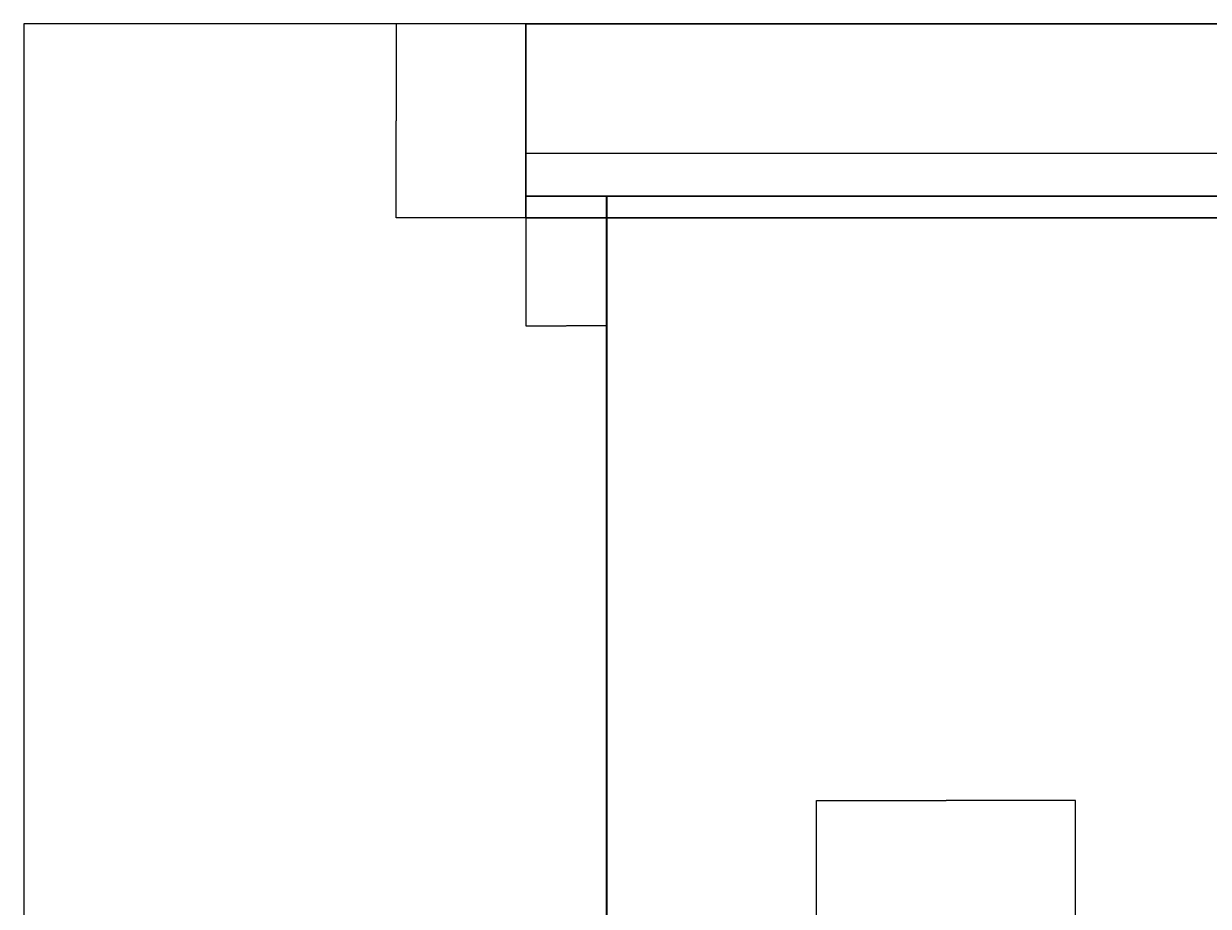
# Model space of a CAD drawing. Units: millimetres. Extents: x 54 to 12356, y 76 to 11627.
# Tile 1 of 2: x 54 to 5541, y 6935 to 11026. Entities that reach past the tile are written whole.
import ezdxf

# ---------------------------------------------------------------- set-up
doc = ezdxf.new("R2010")
doc.units = ezdxf.units.MM
for name, color, linetype, lineweight in [('A-ANNO-DIMS', 2, 'Continuous', 18), ('A-ROOF', 7, 'Continuous', 30), ('A-WALL', 7, 'Continuous', 35)]:
    doc.layers.add(name, color=color, linetype=linetype, lineweight=lineweight)
doc.styles.get("Standard").update_dxf_attribs({"font": 'arial.ttf'})
doc.dimstyles.get("Standard").update_dxf_attribs({"dimtxt": 0.18, "dimasz": 0.18, "dimexe": 0.18, "dimexo": 0.0625, "dimgap": 0.09, "dimtad": 0, "dimtih": 1, "dimtoh": 1, "dimdec": 4, "dimzin": 0, "dimdsep": 46, "dimtxsty": 'Standard', "dimcen": 0.09, "dimadec": 0, "dimazin": 0, "dimtfac": 1, "dimtdec": 4, "dimtofl": 0, "dimtmove": 0, "dimatfit": 3, "dimfxl": 1, "dimtolj": 1, "dimtzin": 0, "dimarcsym": 0})

# ---------------------------------------------------------------- blocks, each defined once
blk = doc.blocks.new('*D20')
at = {"layer": 'A-ANNO-DIMS', "color": 0, "lineweight": -2, "transparency": 16777216}
for p, q in [((2379.868777000001, 11026.423357), (54.25127699999922, 11026.423357)), ((54.43127699999891, 11026.243357), (54.43127700000006, 5851.605321529333)), ((54.43127700000121, 676.6033570000001), (54.43127700000006, 5851.24139247067)), ((654.8687770000003, 676.4233570000002), (54.2512770000013, 676.4233570000001))]:
    blk.add_line(p, q, dxfattribs=at)
at = {"layer": 'A-ANNO-DIMS', "color": 0, "transparency": 16777216}
for points in [[(54.40127699999891, 11026.243357), (54.46127699999891, 11026.243357), (54.43127699999891, 11026.423357)], [(54.40127700000121, 676.6033570000001), (54.46127700000121, 676.6033570000001), (54.43127700000121, 676.4233570000001)]]:
    blk.add_solid(points, dxfattribs=at)
at = {"layer": 'Defpoints', "color": 0, "transparency": 16777216}
for p in [(54.43127699999891, 11026.423357), (2379.931277000001, 11026.423357), (654.9312770000003, 676.4233570000002)]:
    blk.add_point(p, dxfattribs=at)
at = {"layer": 'A-ANNO-DIMS', "color": 0, "transparency": 16777216, "insert": (54.4312770000017, 5851.423357000001), "char_height": 0.18, "attachment_point": 5}
blk.add_mtext('\\A1;10350', dxfattribs=at)
blk = doc.blocks.new('*D21')
at = {"layer": 'A-ANNO-DIMS', "color": 0, "lineweight": -2, "transparency": 16777216}
for p, q in [((2379.931277, 11026.360857), (2379.931277, 10425.743357)), ((11379.931277, 11026.360857), (11379.931277, 10425.743357)), ((2380.111277, 10425.923357), (6879.57281178854, 10425.923357)), ((11379.751277, 10425.923357), (6880.289742211459, 10425.923357))]:
    blk.add_line(p, q, dxfattribs=at)
at = {"layer": 'A-ANNO-DIMS', "color": 0, "transparency": 16777216}
for points in [[(2380.111277, 10425.953357), (2380.111277, 10425.893357), (2379.931277, 10425.923357)], [(11379.751277, 10425.953357), (11379.751277, 10425.893357), (11379.931277, 10425.923357)]]:
    blk.add_solid(points, dxfattribs=at)
at = {"layer": 'Defpoints', "color": 0, "transparency": 16777216}
for p in [(2379.931277, 11026.423357), (11379.931277, 11026.423357), (2379.931277, 10425.923357)]:
    blk.add_point(p, dxfattribs=at)
at = {"layer": 'A-ANNO-DIMS', "color": 0, "transparency": 16777216, "insert": (6879.931277, 10425.923357), "char_height": 0.18, "attachment_point": 5}
blk.add_mtext('\\A1;9000', dxfattribs=at)
blk = doc.blocks.new('*D22')
at = {"layer": 'A-ANNO-DIMS', "color": 0, "lineweight": -2, "transparency": 16777216}
for p, q in [((2379.868777000001, 11026.423357), (1779.251277000001, 11026.423357)), ((1779.431277000001, 11026.243357), (1779.431277000002, 10576.60526013779)), ((1779.431277000002, 10126.603357), (1779.431277000002, 10576.24145386221)), ((2379.868777000001, 10126.423357), (1779.251277000001, 10126.423357))]:
    blk.add_line(p, q, dxfattribs=at)
at = {"layer": 'A-ANNO-DIMS', "color": 0, "transparency": 16777216}
for points in [[(1779.401277000001, 11026.243357), (1779.461277000001, 11026.243357), (1779.431277000001, 11026.423357)], [(1779.401277000002, 10126.603357), (1779.461277000002, 10126.603357), (1779.431277000002, 10126.423357)]]:
    blk.add_solid(points, dxfattribs=at)
at = {"layer": 'Defpoints', "color": 0, "transparency": 16777216}
for p in [(1779.431277000001, 11026.423357), (2379.931277000001, 11026.423357), (2379.931277000001, 10126.423357)]:
    blk.add_point(p, dxfattribs=at)
at = {"layer": 'A-ANNO-DIMS', "color": 0, "transparency": 16777216, "insert": (1779.431277000004, 10576.423357), "char_height": 0.18, "attachment_point": 5}
blk.add_mtext('\\A1;900', dxfattribs=at)
blk = doc.blocks.new('*D23')
at = {"layer": 'A-ANNO-DIMS', "color": 0, "lineweight": -2, "transparency": 16777216}
for p, q in [((2379.931277, 10226.360857), (2379.931277, 9625.743357)), ((2754.931277, 10226.360857), (2754.931277, 9625.743357)), ((2380.111277, 9625.923357), (2567.14181588131, 9625.923357)), ((2754.751277, 9625.923357), (2567.720738118691, 9625.923357))]:
    blk.add_line(p, q, dxfattribs=at)
at = {"layer": 'A-ANNO-DIMS', "color": 0, "transparency": 16777216}
for points in [[(2380.111277, 9625.953357), (2380.111277, 9625.893357), (2379.931277, 9625.923357)], [(2754.751277, 9625.953357), (2754.751277, 9625.893357), (2754.931277, 9625.923357)]]:
    blk.add_solid(points, dxfattribs=at)
at = {"layer": 'Defpoints', "color": 0, "transparency": 16777216}
for p in [(2379.931277, 10226.423357), (2754.931277, 10226.423357), (2379.931277, 9625.923357)]:
    blk.add_point(p, dxfattribs=at)
at = {"layer": 'A-ANNO-DIMS', "color": 0, "transparency": 16777216, "insert": (2567.431277, 9625.923357), "char_height": 0.18, "attachment_point": 5}
blk.add_mtext('\\A1;375', dxfattribs=at)
blk = doc.blocks.new('*D35')
at = {"layer": 'A-ANNO-DIMS', "color": 0, "lineweight": -2, "transparency": 16777216}
for p, q in [((3726.740342, 6825.348683), (3726.740342, 7425.966183000001)), ((3726.920342, 7425.786183000001), (4326.390348821282, 7425.786183000001)), ((4926.560342, 7425.786183000001), (4327.090335178717, 7425.786183000001)), ((4926.740342, 6825.348683), (4926.740342, 7425.966183000001))]:
    blk.add_line(p, q, dxfattribs=at)
at = {"layer": 'A-ANNO-DIMS', "color": 0, "transparency": 16777216}
for points in [[(3726.920342, 7425.816183000001), (3726.920342, 7425.756183), (3726.740342, 7425.786183000001)], [(4926.560342, 7425.816183000001), (4926.560342, 7425.756183), (4926.740342, 7425.786183000001)]]:
    blk.add_solid(points, dxfattribs=at)
at = {"layer": 'Defpoints', "color": 0, "transparency": 16777216}
for p in [(4926.740342, 7425.786183000001), (3726.740342, 6825.286183), (4926.740342, 6825.286183)]:
    blk.add_point(p, dxfattribs=at)
at = {"layer": 'A-ANNO-DIMS', "color": 0, "transparency": 16777216, "insert": (4326.740341999999, 7425.786183000001), "char_height": 0.18, "attachment_point": 5}
blk.add_mtext('\\A1;1200', dxfattribs=at)

msp = doc.modelspace()

# ---------------------------------------------------------------- linework, layer by layer
at = {"layer": 'A-ROOF'}
for p, q in [((2379.931277323882, 10126.42335733614), (2379.931277323882, 11026.42335733614)), ((2379.931277323882, 11026.42335733614), (11379.93127732388, 11026.42335733614)), ((2379.931277323883, 10826.42335733614), (2379.931277323883, 10726.42335733614)), ((11379.93127732388, 10226.42335733614), (2379.931277323882, 10226.42335733614)), ((2379.931277323882, 10126.42335733614), (11004.93127732388, 10126.42335733614))]:
    msp.add_line(p, q, dxfattribs=at)
at = {"layer": 'A-WALL'}
msp.add_line((2754.931277323886, 1276.42335733614), (2754.931277323885, 10226.42335733614), dxfattribs=at)

# ---------------------------------------------------------------- dimensions: what is measured, and where the dimension line sits
at = {"layer": 'A-ANNO-DIMS'}
for base, p1, p2, angle, picture, middle in [((54.43127699999891, 11026.423357), (654.931277, 676.423357), (2379.931277, 11026.423357), 90, '*D20', (54.4312770000017, 5851.423357000001)), ((1779.431277000001, 11026.423357), (2379.931277, 10126.423357), (2379.931277, 11026.423357), 90, '*D22', (1779.431277000004, 10576.423357)), ((2379.931277, 10425.923357), (11379.931277, 11026.423357), (2379.931277, 11026.423357), 180, '*D21', (6879.931277, 10425.923357)), ((2379.931277, 9625.923357), (2754.931277, 10226.423357), (2379.931277, 10226.423357), 180, '*D23', (2567.431277, 9625.923357))]:
    dim = msp.add_linear_dim(base=base, p1=p1, p2=p2, angle=angle, dimstyle='Standard', override={"dimdec": 0, "dimlfac": 1, "dimrnd": 0, "dimzin": 0, "dimdsep": 46, "dimlunit": 2}, dxfattribs=at)
    dim.commit()
    dim.dimension.update_dxf_attribs({"geometry": picture, "text_midpoint": middle})
dim = msp.add_linear_dim(base=(4926.740342, 7425.786183000001), p1=(3726.740342, 6825.286183), p2=(4926.740342, 6825.286183), dimstyle='Standard', override={"dimdec": 0, "dimlfac": 1, "dimrnd": 0, "dimzin": 0, "dimdsep": 46, "dimlunit": 2}, dxfattribs=at)
dim.commit()
dim.dimension.update_dxf_attribs({"geometry": '*D35', "text_midpoint": (4326.740341999999, 7425.786183000001)})

doc.saveas('drawing.dxf')
